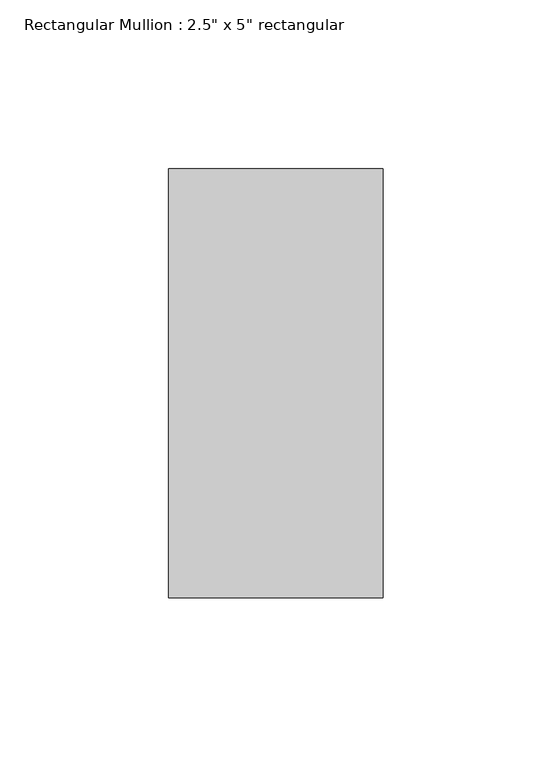
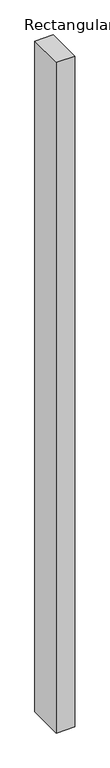
"""IFC4 building model written with IfcOpenShell, lengths in millimetres: member geometry."""

from ifc_helpers import new_model, si_unit, frame, origin, place, context, project, spatial, polyline, outline, extrude, source, transform, mapped, element, save


def member_23836875(model_context):
    return source(origin(), model_context, "Body", "SweptSolid", [
        extrude(outline(polyline([(31.75, 63.5), (31.75, -63.5), (-31.75, -63.5), (-31.75, 63.5), (31.75, 63.5)])), frame((0.0, 0.0, -2440.0217298), z_axis=(0.0, 0.0, 1.0), x_axis=(1.0, 0.0, 0.0)), (0.0, 0.0, 1.0), 2440.0217298),
    ])


if __name__ == "__main__":
    model = new_model("IFC4")
    model_context = context("Model", 3, world=origin())
    ifc_project = project(units=[si_unit("LENGTHUNIT", "METRE", prefix="MILLI")], contexts=[model_context])
    site = spatial("IfcSite", under=ifc_project)
    building = spatial("IfcBuilding", under=site)
    placement = place(None, origin())
    member_shape = member_23836875(model_context)
    element("IfcMember", 1, ObjectType="Rectangular Mullion : 2.5\" x 5\" rectangular", at=placement, inside=building, context=model_context, shape_type="MappedRepresentation", body=[
        mapped(member_shape, transform((0.0, 0.0, 0.0), x_axis=(1.0, 0.0, 0.0), y_axis=(0.0, 1.0, 0.0), z_axis=(0.0, 0.0, 1.0))),
    ])
    save(model, "model.ifc")

# Revit data of these elements
# Type "Rectangular Mullion : 2.5\" x 5\" rectangular"
#   built-in parameter 1007304 = 0.416667 (stored number, unit not read)
#   built-in parameter 1007301 = 0.104167 (stored number, unit not read)
#   built-in parameter 1007300 = 0.104167 (stored number, unit not read)
# Element 1 (IfcMember, "Rectangular Mullion : 2.5\" x 5\" rectangular")
#   Materials on its faces: "Aluminum"
# Materials
#   "Aluminum": class "Metal", colour RGB 247 247 247, transparency 0, Description = "Aluminum 6061", Cost = 0
